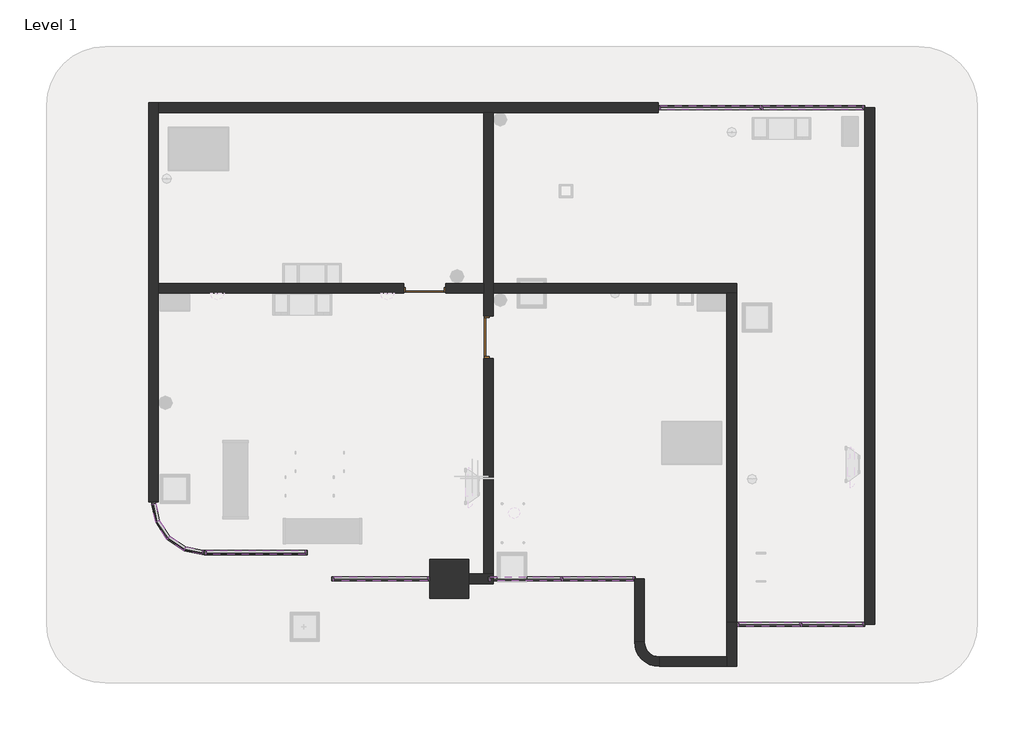
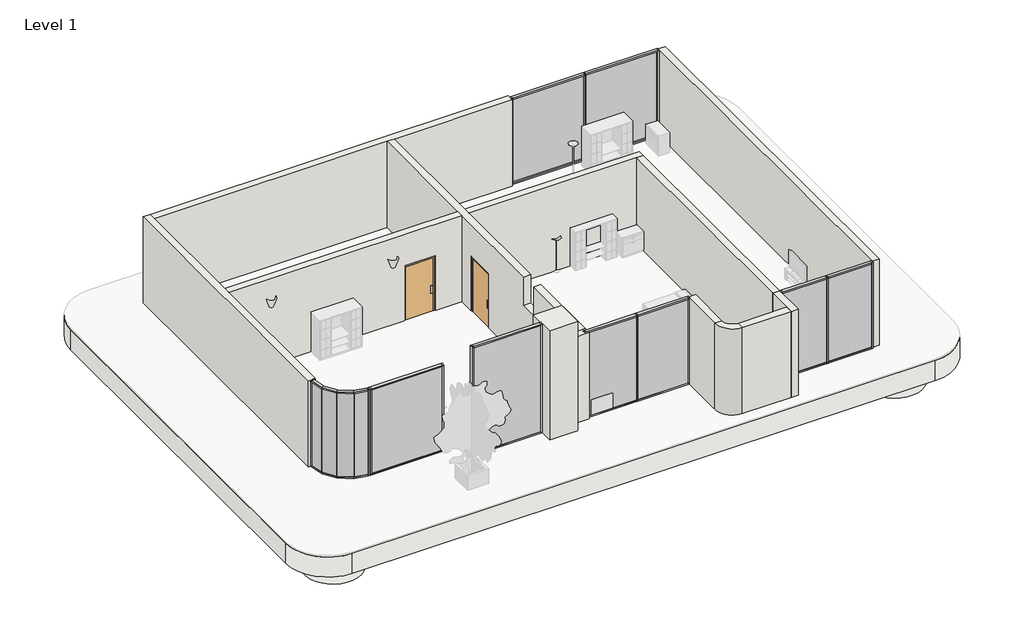
# One storey, part 1 of 2: 39 members, 13 walls, 12 plates, 2 doors, 2 slabs.
"""IFC4 building model written with IfcOpenShell, lengths in millimetres."""

from ifc_helpers import new_model, si_unit, point, frame, frame_2d, origin, origin_with_axes, place, context, project, spatial, polyline, circle_curve, trimmed, segment, composite_curve, outline, extrude, faceted_brep, transform, mapped, element, save
from components import door_bb6275b8, member_c78e4eb6, member_e5c989f4, member_5be86ab4, member_8daf8b49, member_d457d5cf, member_c0191917, member_8659189c, member_c6c1cc64, member_4115b715, member_cd715f5c, member_3783eaa0, system_panel_glazed_b7adf6b9, system_panel_glazed_da3fd9d5, system_panel_glazed_c96b3bd4, system_panel_glazed_89573664, system_panel_glazed_d7bd2e6f, system_panel_glazed_222d0587, system_panel_glazed_285d4db3

model = new_model("IFC4")

# Units and contexts
model_context = context("Model", 3, world=origin())
ifc_project = project(units=[si_unit("LENGTHUNIT", "METRE", prefix="MILLI")], contexts=[model_context])

# Site, building, storey
site = spatial("IfcSite", under=ifc_project)
building = spatial("IfcBuilding", under=site)
storey = spatial("IfcBuildingStorey", under=building, Name="Level 1", Elevation=0.0)

# Doors
placement = place(None, origin())
door_shape = door_bb6275b8(model_context)
element("IfcDoor", 1, ObjectType="Door-Passage-Single-Flush-Dbl_Acting : 48\" x 96\"", at=placement, inside=storey, context=model_context, shape_type="MappedRepresentation", body=[
    mapped(door_shape, transform((-6301.686879, 3653.6091958, 990.6), x_axis=(0.0, 1.0, 0.0), y_axis=(-1.0, 0.0, 0.0), z_axis=(0.0, 0.0, 1.0))),
])
element("IfcDoor", 2, ObjectType="Door-Passage-Single-Flush-Dbl_Acting : 48\" x 96\"", at=placement, inside=storey, context=model_context, shape_type="MappedRepresentation", body=[
    mapped(door_shape, transform((-8289.236879, 5183.9591958, 990.6), x_axis=(-1.0, 0.0, 0.0), y_axis=(0.0, -1.0, 0.0), z_axis=(0.0, 0.0, 1.0))),
])

# Members
member_shape = member_c78e4eb6(model_context)
element("IfcMember", 3, ObjectType="Rectangular Mullion : 2.5\" x 5\" rectangular", at=placement, inside=storey, context=model_context, shape_type="MappedRepresentation", body=[
    mapped(member_shape, transform((1477.063121, -5282.5562261, 4953.0), x_axis=(0.0, 0.0, 1.0), y_axis=(0.0, 1.0, 0.0), z_axis=(-1.0, 0.0, 0.0))),
])
element("IfcMember", 4, ObjectType="Rectangular Mullion : 2.5\" x 5\" rectangular", at=placement, inside=storey, context=model_context, shape_type="MappedRepresentation", body=[
    mapped(member_shape, transform((3437.1390628, -5282.5562261, 4953.0), x_axis=(0.0, 0.0, 1.0), y_axis=(0.0, 1.0, 0.0), z_axis=(-1.0, 0.0, 0.0))),
])
element("IfcMember", 5, ObjectType="Rectangular Mullion : 2.5\" x 5\" rectangular", at=placement, inside=storey, context=model_context, shape_type="MappedRepresentation", body=[
    mapped(member_shape, transform((5333.7150045, -5282.5562261, 990.6), x_axis=(0.0, 0.0, -1.0), y_axis=(0.0, 1.0, 0.0), z_axis=(1.0, 0.0, 0.0))),
])
element("IfcMember", 6, ObjectType="Rectangular Mullion : 2.5\" x 5\" rectangular", at=placement, inside=storey, context=model_context, shape_type="MappedRepresentation", body=[
    mapped(member_shape, transform((3373.6390628, -5282.5562261, 990.6), x_axis=(0.0, 0.0, -1.0), y_axis=(0.0, 1.0, 0.0), z_axis=(1.0, 0.0, 0.0))),
])
member_2_shape = member_e5c989f4(model_context)
element("IfcMember", 7, ObjectType="Rectangular Mullion : 2.5\" x 5\" rectangular", at=placement, inside=storey, context=model_context, shape_type="MappedRepresentation", body=[
    mapped(member_2_shape, transform((3405.3890628, -5282.5562261, 990.6), x_axis=(-1.0, 0.0, 0.0), y_axis=(0.0, 1.0, 0.0), z_axis=(0.0, 0.0, -1.0))),
])
element("IfcMember", 8, ObjectType="Rectangular Mullion : 2.5\" x 5\" rectangular", at=placement, inside=storey, context=model_context, shape_type="MappedRepresentation", body=[
    mapped(member_2_shape, transform((-4022.036879, -3864.7908042, 990.6), x_axis=(-1.0, 0.0, 0.0), y_axis=(0.0, 1.0, 0.0), z_axis=(0.0, 0.0, -1.0))),
])
element("IfcMember", 9, ObjectType="Rectangular Mullion : 2.5\" x 5\" rectangular", at=placement, inside=storey, context=model_context, shape_type="MappedRepresentation", body=[
    mapped(member_2_shape, transform((2184.9997478, 10795.6437739, 990.6), x_axis=(1.0, 0.0, 0.0), y_axis=(0.0, -1.0, 0.0), z_axis=(0.0, 0.0, -1.0))),
])
member_3_shape = member_5be86ab4(model_context)
element("IfcMember", 10, ObjectType="Rectangular Mullion : 2.5\" x 5\" rectangular", at=placement, inside=storey, context=model_context, shape_type="MappedRepresentation", body=[
    mapped(member_3_shape, transform((1413.563121, -5282.5562261, 990.6), x_axis=(-1.0, 0.0, 0.0), y_axis=(0.0, 1.0, 0.0), z_axis=(0.0, 0.0, -1.0))),
])
element("IfcMember", 11, ObjectType="Rectangular Mullion : 2.5\" x 5\" rectangular", at=placement, inside=storey, context=model_context, shape_type="MappedRepresentation", body=[
    mapped(member_3_shape, transform((-6308.036879, -3864.7908042, 990.6), x_axis=(-1.0, 0.0, 0.0), y_axis=(0.0, 1.0, 0.0), z_axis=(0.0, 0.0, -1.0))),
])
element("IfcMember", 12, ObjectType="Rectangular Mullion : 2.5\" x 5\" rectangular", at=placement, inside=storey, context=model_context, shape_type="MappedRepresentation", body=[
    mapped(member_3_shape, transform((5397.2150045, 10795.6437739, 990.6), x_axis=(1.0, 0.0, 0.0), y_axis=(0.0, -1.0, 0.0), z_axis=(0.0, 0.0, -1.0))),
])
element("IfcMember", 13, ObjectType="Rectangular Mullion : 2.5\" x 5\" rectangular", at=placement, inside=storey, context=model_context, shape_type="MappedRepresentation", body=[
    mapped(member_3_shape, transform((-15147.236879, -3051.9908042, 990.6), x_axis=(-1.0, 0.0, 0.0), y_axis=(0.0, 1.0, 0.0), z_axis=(0.0, 0.0, -1.0))),
])
element("IfcMember", 14, ObjectType="Rectangular Mullion : 2.5\" x 5\" rectangular", at=placement, inside=storey, context=model_context, shape_type="MappedRepresentation", body=[
    mapped(member_3_shape, transform((-16724.4155088, -1474.8121743, 990.6), x_axis=(-0.19509032201611579, 0.980785280403233, 0.0), y_axis=(0.980785280403233, 0.19509032201611579, 0.0), z_axis=(0.0, 0.0, -1.0))),
])
element("IfcMember", 15, ObjectType="Rectangular Mullion : 2.5\" x 5\" rectangular", at=placement, inside=storey, context=model_context, shape_type="MappedRepresentation", body=[
    mapped(member_3_shape, transform((5397.2150045, -5282.5562261, 4953.0), x_axis=(1.0, 0.0, 0.0), y_axis=(0.0, 1.0, 0.0), z_axis=(0.0, 0.0, 1.0))),
])
element("IfcMember", 16, ObjectType="Rectangular Mullion : 2.5\" x 5\" rectangular", at=placement, inside=storey, context=model_context, shape_type="MappedRepresentation", body=[
    mapped(member_3_shape, transform((-1736.036879, -3864.7908042, 4953.0), x_axis=(1.0, 0.0, 0.0), y_axis=(0.0, 1.0, 0.0), z_axis=(0.0, 0.0, 1.0))),
])
element("IfcMember", 17, ObjectType="Rectangular Mullion : 2.5\" x 5\" rectangular", at=placement, inside=storey, context=model_context, shape_type="MappedRepresentation", body=[
    mapped(member_3_shape, transform((-1027.2155088, 10795.6437739, 4953.0), x_axis=(-1.0, 0.0, 0.0), y_axis=(0.0, -1.0, 0.0), z_axis=(0.0, 0.0, 1.0))),
])
element("IfcMember", 18, ObjectType="Rectangular Mullion : 2.5\" x 5\" rectangular", at=placement, inside=storey, context=model_context, shape_type="MappedRepresentation", body=[
    mapped(member_3_shape, transform((-11946.836879, -3051.9908042, 4953.0), x_axis=(1.0, 0.0, 0.0), y_axis=(0.0, 1.0, 0.0), z_axis=(0.0, 0.0, 1.0))),
])
element("IfcMember", 19, ObjectType="Rectangular Mullion : 2.5\" x 5\" rectangular", at=placement, inside=storey, context=model_context, shape_type="MappedRepresentation", body=[
    mapped(member_3_shape, transform((-15147.236879, -3051.9908042, 4953.0), x_axis=(0.9807852804032273, -0.19509032201614393, 0.0), y_axis=(0.19509032201614393, 0.9807852804032273, 0.0), z_axis=(0.0, 0.0, 1.0))),
])
member_4_shape = member_8daf8b49(model_context)
element("IfcMember", 20, ObjectType="Rectangular Mullion : 2.5\" x 5\" rectangular", at=placement, inside=storey, context=model_context, shape_type="MappedRepresentation", body=[
    mapped(member_4_shape, transform((-6244.536879, -3864.7908042, 4953.0), x_axis=(0.0, 0.0, 1.0), y_axis=(0.0, 1.0, 0.0), z_axis=(-1.0, 0.0, 0.0))),
])
element("IfcMember", 21, ObjectType="Rectangular Mullion : 2.5\" x 5\" rectangular", at=placement, inside=storey, context=model_context, shape_type="MappedRepresentation", body=[
    mapped(member_4_shape, transform((-3990.286879, -3864.7908042, 4953.0), x_axis=(0.0, 0.0, 1.0), y_axis=(0.0, 1.0, 0.0), z_axis=(-1.0, 0.0, 0.0))),
])
element("IfcMember", 22, ObjectType="Rectangular Mullion : 2.5\" x 5\" rectangular", at=placement, inside=storey, context=model_context, shape_type="MappedRepresentation", body=[
    mapped(member_4_shape, transform((-1799.536879, -3864.7908042, 990.6), x_axis=(0.0, 0.0, -1.0), y_axis=(0.0, 1.0, 0.0), z_axis=(1.0, 0.0, 0.0))),
])
element("IfcMember", 23, ObjectType="Rectangular Mullion : 2.5\" x 5\" rectangular", at=placement, inside=storey, context=model_context, shape_type="MappedRepresentation", body=[
    mapped(member_4_shape, transform((-4053.786879, -3864.7908042, 990.6), x_axis=(0.0, 0.0, -1.0), y_axis=(0.0, 1.0, 0.0), z_axis=(1.0, 0.0, 0.0))),
])
member_5_shape = member_d457d5cf(model_context)
element("IfcMember", 24, ObjectType="Rectangular Mullion : 2.5\" x 5\" rectangular", at=placement, inside=storey, context=model_context, shape_type="MappedRepresentation", body=[
    mapped(member_5_shape, transform((-11121.336879, -3864.7908042, 5994.4), x_axis=(0.0, 0.0, 1.0), y_axis=(0.0, 1.0, 0.0), z_axis=(-1.0, 0.0, 0.0))),
])
element("IfcMember", 25, ObjectType="Rectangular Mullion : 2.5\" x 5\" rectangular", at=placement, inside=storey, context=model_context, shape_type="MappedRepresentation", body=[
    mapped(member_5_shape, transform((-8200.336879, -3864.7908042, 990.6), x_axis=(0.0, 0.0, -1.0), y_axis=(0.0, 1.0, 0.0), z_axis=(1.0, 0.0, 0.0))),
])
member_6_shape = member_c0191917(model_context)
element("IfcMember", 26, ObjectType="Rectangular Mullion : 2.5\" x 5\" rectangular", at=placement, inside=storey, context=model_context, shape_type="MappedRepresentation", body=[
    mapped(member_6_shape, transform((5333.7150045, 10795.6437739, 4953.0), x_axis=(0.0, 0.0, 1.0), y_axis=(0.0, -1.0, 0.0), z_axis=(1.0, 0.0, 0.0))),
])
element("IfcMember", 27, ObjectType="Rectangular Mullion : 2.5\" x 5\" rectangular", at=placement, inside=storey, context=model_context, shape_type="MappedRepresentation", body=[
    mapped(member_6_shape, transform((2153.2497478, 10795.6437739, 4953.0), x_axis=(0.0, 0.0, 1.0), y_axis=(0.0, -1.0, 0.0), z_axis=(1.0, 0.0, 0.0))),
])
element("IfcMember", 28, ObjectType="Rectangular Mullion : 2.5\" x 5\" rectangular", at=placement, inside=storey, context=model_context, shape_type="MappedRepresentation", body=[
    mapped(member_6_shape, transform((-963.7155088, 10795.6437739, 990.6), x_axis=(0.0, 0.0, -1.0), y_axis=(0.0, -1.0, 0.0), z_axis=(-1.0, 0.0, 0.0))),
])
element("IfcMember", 29, ObjectType="Rectangular Mullion : 2.5\" x 5\" rectangular", at=placement, inside=storey, context=model_context, shape_type="MappedRepresentation", body=[
    mapped(member_6_shape, transform((2216.7497478, 10795.6437739, 990.6), x_axis=(0.0, 0.0, -1.0), y_axis=(0.0, -1.0, 0.0), z_axis=(-1.0, 0.0, 0.0))),
])
member_7_shape = member_8659189c(model_context)
element("IfcMember", 30, ObjectType="Rectangular Mullion : 2.5\" x 5\" rectangular", at=placement, inside=storey, context=model_context, shape_type="MappedRepresentation", body=[
    mapped(member_7_shape, transform((-16712.0272734, -1537.0920396, 4953.0), x_axis=(0.0, 0.0, 1.0), y_axis=(0.980785280403233, 0.19509032201611579, 0.0), z_axis=(-0.19509032201611579, 0.980785280403233, 0.0))),
])
member_8_shape = member_c6c1cc64(model_context)
element("IfcMember", 31, ObjectType="Rectangular Mullion : 2.5\" x 5\" rectangular", at=placement, inside=storey, context=model_context, shape_type="MappedRepresentation", body=[
    mapped(member_8_shape, transform((-16262.4705833, -2590.0458786, 990.6), x_axis=(0.0, 0.0, -1.0), y_axis=(0.8314696123025568, 0.5555702330195851, 0.0), z_axis=(0.555570233019585, -0.8314696123025567, 0.0))),
])
element("IfcMember", 32, ObjectType="Rectangular Mullion : 2.5\" x 5\" rectangular", at=placement, inside=storey, context=model_context, shape_type="MappedRepresentation", body=[
    mapped(member_8_shape, transform((-16604.3599342, -2078.3723059, 4953.0), x_axis=(0.0, 0.0, 1.0), y_axis=(0.831469612302557, 0.5555702330195846, 0.0), z_axis=(-0.5555702330195846, 0.831469612302557, 0.0))),
])
member_9_shape = member_4115b715(model_context)
element("IfcMember", 33, ObjectType="Rectangular Mullion : 2.5\" x 5\" rectangular", at=placement, inside=storey, context=model_context, shape_type="MappedRepresentation", body=[
    mapped(member_9_shape, transform((-16604.3599342, -2078.3723059, 990.6), x_axis=(0.0, 0.0, -1.0), y_axis=(0.980785280403233, 0.19509032201611579, 0.0), z_axis=(0.19509032201611579, -0.980785280403233, 0.0))),
])
member_10_shape = member_cd715f5c(model_context)
element("IfcMember", 34, ObjectType="Rectangular Mullion : 2.5\" x 5\" rectangular", at=placement, inside=storey, context=model_context, shape_type="MappedRepresentation", body=[
    mapped(member_10_shape, transform((-11184.836879, -3864.7908042, 990.6), x_axis=(-1.0, 0.0, 0.0), y_axis=(0.0, 1.0, 0.0), z_axis=(0.0, 0.0, -1.0))),
])
element("IfcMember", 35, ObjectType="Rectangular Mullion : 2.5\" x 5\" rectangular", at=placement, inside=storey, context=model_context, shape_type="MappedRepresentation", body=[
    mapped(member_10_shape, transform((-8136.836879, -3864.7908042, 5994.4), x_axis=(1.0, 0.0, 0.0), y_axis=(0.0, 1.0, 0.0), z_axis=(0.0, 0.0, 1.0))),
])
element("IfcMember", 36, ObjectType="Rectangular Mullion : 2.5\" x 5\" rectangular", at=placement, inside=storey, context=model_context, shape_type="MappedRepresentation", body=[
    mapped(member_8_shape, transform((-16262.4705833, -2590.0458786, 4953.0), x_axis=(0.0, 0.0, 1.0), y_axis=(0.5555702330196194, 0.8314696123025339, 0.0), z_axis=(-0.8314696123025338, 0.5555702330196193, 0.0))),
])
element("IfcMember", 37, ObjectType="Rectangular Mullion : 2.5\" x 5\" rectangular", at=placement, inside=storey, context=model_context, shape_type="MappedRepresentation", body=[
    mapped(member_8_shape, transform((-15750.7970105, -2931.9352296, 990.6), x_axis=(0.0, 0.0, -1.0), y_axis=(0.5555702330196189, 0.8314696123025341, 0.0), z_axis=(0.831469612302534, -0.5555702330196188, 0.0))),
])
element("IfcMember", 38, ObjectType="Rectangular Mullion : 2.5\" x 5\" rectangular", at=placement, inside=storey, context=model_context, shape_type="MappedRepresentation", body=[
    mapped(member_7_shape, transform((-15209.5167443, -3039.6025687, 990.6), x_axis=(0.0, 0.0, -1.0), y_axis=(0.19509032201614393, 0.9807852804032273, 0.0), z_axis=(0.9807852804032272, -0.1950903220161439, 0.0))),
])
element("IfcMember", 39, ObjectType="Rectangular Mullion : 2.5\" x 5\" rectangular", at=placement, inside=storey, context=model_context, shape_type="MappedRepresentation", body=[
    mapped(member_9_shape, transform((-15750.7970105, -2931.9352296, 4953.0), x_axis=(0.0, 0.0, 1.0), y_axis=(0.19509032201614393, 0.9807852804032273, 0.0), z_axis=(-0.9807852804032272, 0.1950903220161439, 0.0))),
])
member_11_shape = member_3783eaa0(model_context)
element("IfcMember", 40, ObjectType="Rectangular Mullion : 2.5\" x 5\" rectangular", at=placement, inside=storey, context=model_context, shape_type="MappedRepresentation", body=[
    mapped(member_11_shape, transform((-15083.736879, -3051.9908042, 4953.0), x_axis=(0.0, 0.0, 1.0), y_axis=(0.0, 1.0, 0.0), z_axis=(-1.0, 0.0, 0.0))),
])
element("IfcMember", 41, ObjectType="Rectangular Mullion : 2.5\" x 5\" rectangular", at=placement, inside=storey, context=model_context, shape_type="MappedRepresentation", body=[
    mapped(member_11_shape, transform((-12010.336879, -3051.9908042, 990.6), x_axis=(0.0, 0.0, -1.0), y_axis=(0.0, 1.0, 0.0), z_axis=(1.0, 0.0, 0.0))),
])

# Plates
system_panel_glazed_shape = system_panel_glazed_b7adf6b9(model_context)
element("IfcPlate", 42, ObjectType="System Panel : Glazed", at=placement, inside=storey, context=model_context, shape_type="MappedRepresentation", body=[
    mapped(system_panel_glazed_shape, transform((4385.4270336, -5282.5562261, 1054.1), x_axis=(-1.0, 0.0, 0.0), y_axis=(0.0, -1.0, 0.0), z_axis=(0.0, 0.0, 1.0))),
])
element("IfcPlate", 43, ObjectType="System Panel : Glazed", at=placement, inside=storey, context=model_context, shape_type="MappedRepresentation", body=[
    mapped(system_panel_glazed_shape, transform((2425.3510919, -5282.5562261, 1054.1), x_axis=(-1.0, 0.0, 0.0), y_axis=(0.0, -1.0, 0.0), z_axis=(0.0, 0.0, 1.0))),
])
system_panel_glazed_2_shape = system_panel_glazed_da3fd9d5(model_context)
element("IfcPlate", 44, ObjectType="System Panel : Glazed", at=placement, inside=storey, context=model_context, shape_type="MappedRepresentation", body=[
    mapped(system_panel_glazed_2_shape, transform((-2894.911879, -3864.7908042, 1054.1), x_axis=(-1.0, 0.0, 0.0), y_axis=(0.0, -1.0, 0.0), z_axis=(0.0, 0.0, 1.0))),
])
element("IfcPlate", 45, ObjectType="System Panel : Glazed", at=placement, inside=storey, context=model_context, shape_type="MappedRepresentation", body=[
    mapped(system_panel_glazed_2_shape, transform((-5149.161879, -3864.7908042, 1054.1), x_axis=(-1.0, 0.0, 0.0), y_axis=(0.0, -1.0, 0.0), z_axis=(0.0, 0.0, 1.0))),
])
system_panel_glazed_3_shape = system_panel_glazed_c96b3bd4(model_context)
element("IfcPlate", 46, ObjectType="System Panel : Glazed", at=placement, inside=storey, context=model_context, shape_type="MappedRepresentation", body=[
    mapped(system_panel_glazed_3_shape, transform((594.7671195, 10795.6437739, 1054.1), x_axis=(1.0, 0.0, 0.0), y_axis=(0.0, 1.0, 0.0), z_axis=(0.0, 0.0, 1.0))),
])
element("IfcPlate", 47, ObjectType="System Panel : Glazed", at=placement, inside=storey, context=model_context, shape_type="MappedRepresentation", body=[
    mapped(system_panel_glazed_3_shape, transform((3775.2323762, 10795.6437739, 1054.1), x_axis=(1.0, 0.0, 0.0), y_axis=(0.0, 1.0, 0.0), z_axis=(0.0, 0.0, 1.0))),
])
system_panel_glazed_4_shape = system_panel_glazed_89573664(model_context)
element("IfcPlate", 48, ObjectType="System Panel : Glazed", at=placement, inside=storey, context=model_context, shape_type="MappedRepresentation", body=[
    mapped(system_panel_glazed_4_shape, transform((-15480.1568774, -2985.7688991, 1054.1), x_axis=(-0.9807852804032273, 0.19509032201614393, 0.0), y_axis=(-0.19509032201614393, -0.9807852804032273, 0.0), z_axis=(0.0, 0.0, 1.0))),
])
element("IfcPlate", 49, ObjectType="System Panel : Glazed", at=placement, inside=storey, context=model_context, shape_type="MappedRepresentation", body=[
    mapped(system_panel_glazed_4_shape, transform((-16658.1936038, -1807.7321727, 1054.1), x_axis=(-0.19509032201611579, 0.980785280403233, 0.0), y_axis=(-0.980785280403233, -0.19509032201611579, 0.0), z_axis=(0.0, 0.0, 1.0))),
])
system_panel_glazed_5_shape = system_panel_glazed_d7bd2e6f(model_context)
element("IfcPlate", 50, ObjectType="System Panel : Glazed", at=placement, inside=storey, context=model_context, shape_type="MappedRepresentation", body=[
    mapped(system_panel_glazed_5_shape, transform((-16433.4152587, -2334.2090922, 1054.1), x_axis=(-0.5555702330195851, 0.8314696123025568, 0.0), y_axis=(-0.8314696123025568, -0.5555702330195851, 0.0), z_axis=(0.0, 0.0, 1.0))),
])
element("IfcPlate", 51, ObjectType="System Panel : Glazed", at=placement, inside=storey, context=model_context, shape_type="MappedRepresentation", body=[
    mapped(system_panel_glazed_5_shape, transform((-16006.6337969, -2760.9905541, 1054.1), x_axis=(-0.8314696123025341, 0.5555702330196189, 0.0), y_axis=(-0.5555702330196189, -0.8314696123025341, 0.0), z_axis=(0.0, 0.0, 1.0))),
])
system_panel_glazed_6_shape = system_panel_glazed_222d0587(model_context)
element("IfcPlate", 52, ObjectType="System Panel : Glazed", at=placement, inside=storey, context=model_context, shape_type="MappedRepresentation", body=[
    mapped(system_panel_glazed_6_shape, transform((-9660.836879, -3864.7908042, 1054.1), x_axis=(-1.0, 0.0, 0.0), y_axis=(0.0, -1.0, 0.0), z_axis=(0.0, 0.0, 1.0))),
])
system_panel_glazed_7_shape = system_panel_glazed_285d4db3(model_context)
element("IfcPlate", 53, ObjectType="System Panel : Glazed", at=placement, inside=storey, context=model_context, shape_type="MappedRepresentation", body=[
    mapped(system_panel_glazed_7_shape, transform((-13547.036879, -3051.9908042, 1054.1), x_axis=(-1.0, 0.0, 0.0), y_axis=(0.0, -1.0, 0.0), z_axis=(0.0, 0.0, 1.0))),
])

# Slabs
element("IfcSlab", 54, ObjectType="Generic - 3'", at=placement, inside=storey, context=model_context, shape_type="SweptSolid", body=[
    extrude(outline(composite_curve([segment(trimmed(circle_curve(frame_2d((7073.6150045, 10871.8437739)), 1828.8), [point((7073.6150045, 12700.6437739))], [point((8902.4150045, 10871.8437739))], False, "CARTESIAN"), True, "CONTINUOUS"), segment(polyline([(8902.4150045, 10871.8437739), (8902.4150045, -5282.5562261)]), True, "CONTINUOUS"), segment(trimmed(circle_curve(frame_2d((7073.6150045, -5282.5562261)), 1828.8), [point((8902.4150045, -5282.5562261))], [point((7073.6150045, -7111.3562261))], False, "CARTESIAN"), True, "CONTINUOUS"), segment(polyline([(7073.6150045, -7111.3562261), (-18224.7849955, -7111.3562261)]), True, "CONTINUOUS"), segment(trimmed(circle_curve(frame_2d((-18224.7849955, -5282.5562261)), 1828.8), [point((-18224.7849955, -7111.3562261))], [point((-20053.5849955, -5282.5562261))], False, "CARTESIAN"), True, "CONTINUOUS"), segment(polyline([(-20053.5849955, -5282.5562261), (-20053.5849955, 10871.8437739)]), True, "CONTINUOUS"), segment(trimmed(circle_curve(frame_2d((-18224.7849955, 10871.8437739)), 1828.8), [point((-20053.5849955, 10871.8437739))], [point((-18224.7849955, 12700.6437739))], False, "CARTESIAN"), True, "CONTINUOUS"), segment(polyline([(-18224.7849955, 12700.6437739), (7073.6150045, 12700.6437739)]), True, "CONTINUOUS")], self_intersect=False)), origin_with_axes(), (0.0, 0.0, 1.0), 914.4),
])
element("IfcSlab", 55, ObjectType="Generic - 4'", at=placement, inside=storey, context=model_context, shape_type="SweptSolid", body=[
    extrude(outline(composite_curve([segment(trimmed(circle_curve(frame_2d((6642.5508629, 10443.6424497)), 1219.2), [point((5423.3508629, 10443.6424497))], [point((6642.5508629, 9224.4424497))], False, "CARTESIAN"), True, "CONTINUOUS"), segment(polyline([(6642.5508629, 9224.4424497), (6642.5508629, -3577.1575503)]), True, "CONTINUOUS"), segment(trimmed(circle_curve(frame_2d((6642.5508629, -4796.3575503)), 1219.2), [point((6642.5508629, -3577.1575503))], [point((5423.3508629, -4796.3575503))], False, "CARTESIAN"), True, "CONTINUOUS"), segment(polyline([(5423.3508629, -4796.3575503), (-16522.2491371, -4796.3575503)]), True, "CONTINUOUS"), segment(trimmed(circle_curve(frame_2d((-17741.4491371, -4796.3575503)), 1219.2), [point((-16522.2491371, -4796.3575503))], [point((-17741.4491371, -3577.1575503))], False, "CARTESIAN"), True, "CONTINUOUS"), segment(polyline([(-17741.4491371, -3577.1575503), (-17741.4491371, 9224.4424497)]), True, "CONTINUOUS"), segment(trimmed(circle_curve(frame_2d((-17741.4491371, 10443.6424497)), 1219.2), [point((-17741.4491371, 9224.4424497))], [point((-16522.2491371, 10443.6424497))], False, "CARTESIAN"), True, "CONTINUOUS"), segment(polyline([(-16522.2491371, 10443.6424497), (5423.3508629, 10443.6424497)]), True, "CONTINUOUS")], self_intersect=False)), frame((0.0, 0.0, -1219.2), z_axis=(0.0, 0.0, 1.0), x_axis=(1.0, 0.0, 0.0)), (0.0, 0.0, 1.0), 1219.2),
])

# Walls
element("IfcWall", 56, ObjectType="Generic - 12\"", at=placement, inside=storey, context=model_context, shape_type="Brep", body=[
    faceted_brep([(1108.763121, -5225.9294098, 990.6), (1108.763121, -6292.7294098, 990.6), (1108.763121, -6597.5294098, 990.6), (1108.763121, -6597.5294098, 4953.0), (1108.763121, -6292.7294098, 4953.0), (1108.763121, -5225.9294098, 4953.0), (1413.563121, -5225.9294098, 990.6), (1413.563121, -5225.9294098, 4953.0), (1413.563121, -6597.5294098, 4953.0), (1413.563121, -6597.5294098, 990.6)], [[[0, 1, 2, 3, 4, 5]], [[6, 7, 8, 9]], [[2, 1, 0, 6, 9]], [[5, 4, 3, 8, 7]], [[0, 5, 7, 6]], [[3, 2, 9, 8]]]),
])
element("IfcWall", 57, ObjectType="Generic - 12\"", at=placement, inside=storey, context=model_context, shape_type="SweptSolid", body=[
    extrude(outline(polyline([(-999.436879, -6292.7294098), (1108.763121, -6292.7294098), (1108.763121, -6597.5294098), (-999.436879, -6597.5294098), (-999.436879, -6292.7294098)])), frame((0.0, 0.0, 990.6), z_axis=(0.0, 0.0, 1.0), x_axis=(1.0, 0.0, 0.0)), (0.0, 0.0, 1.0), 3962.4),
])
element("IfcWall", 58, ObjectType="Generic - 12\"", at=placement, inside=storey, context=model_context, shape_type="SweptSolid", body=[
    extrude(outline(polyline([(-1456.636879, -3864.7908042), (-1456.636879, -5835.5294098), (-1761.436879, -5835.5294098), (-1761.436879, -3864.7908042), (-1456.636879, -3864.7908042)])), frame((0.0, 0.0, 990.6), z_axis=(0.0, 0.0, 1.0), x_axis=(1.0, 0.0, 0.0)), (0.0, 0.0, 1.0), 3962.4),
])
element("IfcWall", 59, ObjectType="Generic - 12\"", at=placement, inside=storey, context=model_context, shape_type="SweptSolid", body=[
    extrude(outline(composite_curve([segment(polyline([(-999.436879, -6292.7294098), (-999.436879, -6597.5294098)]), True, "CONTINUOUS"), segment(trimmed(circle_curve(frame_2d((-999.436879, -5835.5294098)), 762.0), [point((-999.436879, -6597.5294098))], [point((-1761.436879, -5835.5294098))], False, "CARTESIAN"), True, "CONTINUOUS"), segment(polyline([(-1761.436879, -5835.5294098), (-1456.636879, -5835.5294098)]), True, "CONTINUOUS"), segment(trimmed(circle_curve(frame_2d((-999.436879, -5835.5294098)), 457.2), [point((-1456.636879, -5835.5294098))], [point((-999.436879, -6292.7294098))], True, "CARTESIAN"), True, "CONTINUOUS")], self_intersect=False)), frame((0.0, 0.0, 990.6), z_axis=(0.0, 0.0, 1.0), x_axis=(1.0, 0.0, 0.0)), (0.0, 0.0, 1.0), 3962.4),
])
element("IfcWall", 60, ObjectType="Generic - 12\"", at=placement, inside=storey, context=model_context, shape_type="Brep", body=[
    faceted_brep([(-6155.636879, -3712.3908042, 990.6), (-6460.436879, -3712.3908042, 990.6), (-6917.636879, -3712.3908042, 990.6), (-6917.636879, -3712.3908042, 4953.0), (-6460.436879, -3712.3908042, 4953.0), (-6155.636879, -3712.3908042, 4953.0), (-6155.636879, -4017.1908042, 990.6), (-6155.636879, -4017.1908042, 4953.0), (-6917.636879, -4017.1908042, 4953.0), (-6917.636879, -4017.1908042, 990.6)], [[[0, 1, 2, 3, 4, 5]], [[6, 7, 8, 9]], [[2, 1, 0, 6, 9]], [[3, 2, 9, 8]], [[5, 4, 3, 8, 7]], [[0, 5, 7, 6]]]),
])
element("IfcWall", 61, ObjectType="Generic - 12\"", at=placement, inside=storey, context=model_context, shape_type="Brep", body=[
    faceted_brep([(-6155.636879, -3712.3908042, 4953.0), (-6155.636879, -3712.3908042, 990.6), (-6155.636879, 2993.2091958, 990.6), (-6155.636879, 2993.2091958, 3530.6), (-6155.636879, 4314.0091958, 3530.6), (-6155.636879, 4314.0091958, 990.6), (-6155.636879, 5025.2091958, 990.6), (-6155.636879, 5330.0091958, 990.6), (-6155.636879, 10643.2437739, 990.6), (-6155.636879, 10643.2437739, 4953.0), (-6155.636879, 5330.0091958, 4953.0), (-6155.636879, 5025.2091958, 4953.0), (-6155.636879, 377.0091958, 4953.0), (-6155.636879, 377.0091958, 3648.2722241), (-6155.636879, -384.9908042, 3648.2722241), (-6155.636879, -384.9908042, 4953.0), (-6460.436879, -3712.3908042, 990.6), (-6460.436879, -3712.3908042, 4953.0), (-6460.436879, -384.9908042, 4953.0), (-6460.436879, -384.9908042, 3648.2722241), (-6460.436879, 377.0091958, 3648.2722241), (-6460.436879, 377.0091958, 4953.0), (-6460.436879, 5025.2091958, 4953.0), (-6460.436879, 5330.0091958, 4953.0), (-6460.436879, 10643.2437739, 4953.0), (-6460.436879, 10643.2437739, 990.6), (-6460.436879, 5330.0091958, 990.6), (-6460.436879, 5025.2091958, 990.6), (-6460.436879, 4314.0091958, 990.6), (-6460.436879, 4314.0091958, 3530.6), (-6460.436879, 2993.2091958, 3530.6), (-6460.436879, 2993.2091958, 990.6)], [[[0, 1, 2, 3, 4, 5, 6, 7, 8, 9, 10, 11, 12, 13, 14, 15]], [[16, 17, 18, 19, 20, 21, 22, 23, 24, 25, 26, 27, 28, 29, 30, 31]], [[1, 16, 31, 2]], [[25, 8, 7, 6, 5, 28, 27, 26]], [[17, 0, 15, 18]], [[9, 24, 23, 22, 21, 12, 11, 10]], [[1, 0, 17, 16]], [[9, 8, 25, 24]], [[4, 29, 28, 5]], [[29, 4, 3, 30]], [[30, 3, 2, 31]], [[14, 19, 18, 15]], [[19, 14, 13, 20]], [[20, 13, 12, 21]]]),
])
element("IfcWall", 62, ObjectType="Generic - 12\"", at=placement, inside=storey, context=model_context, shape_type="Brep", body=[
    faceted_brep([(-6155.636879, 5025.2091958, 990.6), (1108.763121, 5025.2091958, 990.6), (1413.563121, 5025.2091958, 990.6), (1413.563121, 5025.2091958, 4953.0), (1108.763121, 5025.2091958, 4953.0), (-6155.636879, 5025.2091958, 4953.0), (-6155.636879, 5330.0091958, 990.6), (-6155.636879, 5330.0091958, 4953.0), (1413.563121, 5330.0091958, 4953.0), (1413.563121, 5330.0091958, 990.6)], [[[0, 1, 2, 3, 4, 5]], [[6, 7, 8, 9]], [[2, 1, 0, 6, 9]], [[5, 4, 3, 8, 7]], [[0, 5, 7, 6]], [[3, 2, 9, 8]]]),
])
element("IfcWall", 63, ObjectType="Generic - 12\"", at=placement, inside=storey, context=model_context, shape_type="SweptSolid", body=[
    extrude(outline(polyline([(1108.763121, -5225.9294098), (1108.763121, 5025.2091958), (1413.563121, 5025.2091958), (1413.563121, -5225.9294098), (1108.763121, -5225.9294098)])), frame((0.0, 0.0, 990.6), z_axis=(0.0, 0.0, 1.0), x_axis=(1.0, 0.0, 0.0)), (0.0, 0.0, 1.0), 3962.4),
])
element("IfcWall", 64, ObjectType="Generic - 12\"", at=placement, inside=storey, context=model_context, shape_type="SweptSolid", body=[
    extrude(outline(polyline([(4953.0, -6460.436879), (4953.0, -16572.0155088), (990.6, -16572.0155088), (990.6, -8949.636879), (3530.6, -8949.636879), (3530.6, -7628.836879), (990.6, -7628.836879), (990.6, -6460.436879), (4953.0, -6460.436879)])), frame((0.0, 5025.2091958, 0.0), z_axis=(0.0, 1.0, 0.0), x_axis=(0.0, 0.0, 1.0)), (0.0, 0.0, 1.0), 304.8),
])
element("IfcWall", 65, ObjectType="Generic - 12\" yellow", at=placement, inside=storey, context=model_context, shape_type="Brep", body=[
    faceted_brep([(-16572.0155088, -1474.8121743, 990.6), (-16572.0155088, 5025.2091958, 990.6), (-16572.0155088, 5330.0091958, 990.6), (-16572.0155088, 10643.2437739, 990.6), (-16572.0155088, 10948.0437739, 990.6), (-16572.0155088, 10948.0437739, 4953.0), (-16572.0155088, 10643.2437739, 4953.0), (-16572.0155088, 5330.0091958, 4953.0), (-16572.0155088, 5025.2091958, 4953.0), (-16572.0155088, -1474.8121743, 4953.0), (-16876.8155088, -1474.8121743, 990.6), (-16876.8155088, -1474.8121743, 4953.0), (-16876.8155088, 10948.0437739, 4953.0), (-16876.8155088, 10948.0437739, 990.6)], [[[0, 1, 2, 3, 4, 5, 6, 7, 8, 9]], [[10, 11, 12, 13]], [[4, 3, 2, 1, 0, 10, 13]], [[9, 8, 7, 6, 5, 12, 11]], [[0, 9, 11, 10]], [[5, 4, 13, 12]]]),
])
element("IfcWall", 66, ObjectType="Generic - 12\" yellow", at=placement, inside=storey, context=model_context, shape_type="SweptSolid", body=[
    extrude(outline(polyline([(5702.0150045, 10795.6437739), (5702.0150045, -5282.5562261), (5397.2150045, -5282.5562261), (5397.2150045, 10795.6437739), (5702.0150045, 10795.6437739)])), frame((0.0, 0.0, 990.6), z_axis=(0.0, 0.0, 1.0), x_axis=(1.0, 0.0, 0.0)), (0.0, 0.0, 1.0), 3962.4),
])
element("IfcWall", 67, ObjectType="Generic - 12\" yellow", at=placement, inside=storey, context=model_context, shape_type="Brep", body=[
    faceted_brep([(-16572.0155088, 10643.2437739, 990.6), (-6460.436879, 10643.2437739, 990.6), (-6155.636879, 10643.2437739, 990.6), (-1027.2155088, 10643.2437739, 990.6), (-1027.2155088, 10643.2437739, 4953.0), (-6155.636879, 10643.2437739, 4953.0), (-6460.436879, 10643.2437739, 4953.0), (-16572.0155088, 10643.2437739, 4953.0), (-16572.0155088, 10948.0437739, 990.6), (-16572.0155088, 10948.0437739, 4953.0), (-1027.2155088, 10948.0437739, 4953.0), (-1027.2155088, 10948.0437739, 990.6)], [[[0, 1, 2, 3, 4, 5, 6, 7]], [[8, 9, 10, 11]], [[3, 2, 1, 0, 8, 11]], [[4, 3, 11, 10]], [[7, 6, 5, 4, 10, 9]], [[0, 7, 9, 8]]]),
])
element("IfcWall", 68, ObjectType="Generic - 7'", at=placement, inside=storey, context=model_context, shape_type="Brep", body=[
    faceted_brep([(-6917.636879, -3255.1908042, 990.6), (-8136.836879, -3255.1908042, 990.6), (-8136.836879, -3255.1908042, 5994.4), (-6917.636879, -3255.1908042, 5994.4), (-6917.636879, -4474.3908042, 990.6), (-6917.636879, -4474.3908042, 5994.4), (-8136.836879, -4474.3908042, 5994.4), (-8136.836879, -4474.3908042, 990.6), (-6917.636879, -3712.3908042, 990.6), (-6917.636879, -4017.1908042, 990.6)], [[[0, 1, 2, 3]], [[4, 5, 6, 7]], [[1, 0, 8, 9, 4, 7]], [[2, 1, 7, 6]], [[3, 2, 6, 5]], [[0, 3, 5, 4, 9, 8]]]),
])

save(model, "model.ifc")

# Revit data of these elements
# Type "Door-Passage-Single-Flush-Dbl_Acting : 48\" x 96\""
#   Type Mark = "8"
#   Assembly Code = "B2030200"
#   Analytic Construction = "Wooden"
#   Thickness = 0' - 1 3/4"
#   Thermal Resistance (R) = 2.5876 (h·ft²·°F)/BTU
#   Swing Angle [instance default] = 45.00°
#   Strike Height = 3' - 4"
#   Rough Width [instance default] = 4' - 4"
#   Rough Height [instance default] = 8' - 4"
#   MF Opening Height [instance default] = 0' - 4"
#   MF Opening Width [instance default] = 0' - 4"
#   Inset Calculate [instance default] = 0' - 4"
#   Masonry Inset [instance default] = 0' - 1"
#   Height = 8' - 0"
#   Width = 4' - 0"
#   Heat Transfer Coefficient (U) = 0.3865 BTU/(h·ft²·°F)
#   Masonry Frame Depth = 0' - 5 3/4"
#   Masonry Frame [instance default] = yes
#   Function = 1
#   Dry Wall Frame [instance default] = no
#   Panel Material = Wood - Birch
#   Frame Material = Metal - Paint Finish - Grey
#   Door Handle Material = Aluminum
#   Visual Light Transmittance = 0
#   Solar Heat Gain Coefficient = 0
#   Wall Closure = (empty or 0)
# Type "Rectangular Mullion : 2.5\" x 5\" rectangular"
#   built-in parameter 1007304 = 0.416667 (stored number, unit not read)
#   built-in parameter 1007301 = 0.104167 (stored number, unit not read)
#   built-in parameter 1007300 = 0.104167 (stored number, unit not read)
# Type "System Panel : Glazed"
#   Construction Type Id = "GSP4R"
#   Analytic Construction = "1/8 in Pilkington single glazing"
#   Visual Light Transmittance = 0.9
#   Solar Heat Gain Coefficient = 0.86
#   Heat Transfer Coefficient (U) = 1.18115 BTU/(h·ft²·°F)
# Type "Generic - 3'"
#   Assembly Code = "B1010"
#   Function = 0
#   Layers, outside or top first: 3' - 0" "Parking Stripe" (function 1)
# Type "Generic - 4'"
#   Assembly Code = "B1010"
#   Function = 0
#   Layers, outside or top first: 4' - 0" "Parking Stripe" (function 1)
# Type "Generic - 12\""
#   Assembly Code = "B2010"
#   Layers, outside or top first: 1' - 0" "Parking Stripe" (function 1)
# Type "Generic - 12\" yellow"
#   Assembly Code = "B2010"
#   Layers, outside or top first: 1' - 0" "Door - Frame" (function 1)
# Type "Generic - 7'"
#   Assembly Code = "B2010"
#   Layers, outside or top first: 4' - 0" "Parking Stripe" (function 1)
# Elements 1, 2 (IfcDoor, "Door-Passage-Single-Flush-Dbl_Acting : 48\" x 96\"")
#   Swing Angle = 45.00°
#   Rough Width = 4' - 4"
#   Rough Height = 8' - 4"
#   Masonry Inset = 0' - 1"
#   MF Opening Width = 0' - 4"
#   MF Opening Height = 0' - 4"
#   Inset Calculate = 0' - 4"
#   Masonry Frame = yes
#   Dry Wall Frame = no
#   Phase Created = New Construction
#   Materials on its faces: "Aluminum", "Metal - Paint Finish - Grey", "Wood - Birch"
# Elements 3, 4, 5, 6, 7, 8, 9, 10, 11, 12, 13, 14, 15, 16, 17, 18, 19, 20, 21, 22, 23, 24, 25, 26, 27, 28, 29, 30, 31, 32, 33, 34, 35, 36, 37, 38, 39, 40, 41 (IfcMember, "Rectangular Mullion : 2.5\" x 5\" rectangular")
#   Phase Created = New Construction
#   Materials on its faces: "Iron, Ductile"
# Elements 42, 43, 44, 45, 46, 47, 48, 49, 50, 51, 52, 53 (IfcPlate, "System Panel : Glazed")
#   Phase Created = New Construction
#   Materials on its faces: "Glass"
# Element 54 (IfcSlab, "Generic - 3'")
#   Height Offset From Level = 3' - 0"
#   Phase Created = New Construction
#   Materials on its faces: "Parking Stripe"
# Element 55 (IfcSlab, "Generic - 4'")
#   Height Offset From Level = 0' - 0"
#   Phase Created = New Construction
#   Materials on its faces: "Parking Stripe"
# Element 56 (IfcWall, "Generic - 12\"")
#   built-in parameter 1001111 = 3' - 3"
#   Top Offset = 0' - 0"
#   Base Offset = 3' - 3"
#   Unconnected Height = 13' - 0"
#   wall height = 13' - 0"
#   Phase Created = New Construction
#   Base Constraint = Level 1
#   Materials on its faces: "Parking Stripe"
# Elements 57, 58, 60, 61, 63, 64 (IfcWall, "Generic - 12\"")
#   built-in parameter 1001111 = 3' - 3"
#   Top Offset = 0' - 0"
#   Base Offset = 3' - 3"
#   Unconnected Height = 13' - 0"
#   wall height = 13' - 0"
#   Phase Created = New Construction
#   Base Constraint = Level 1
#   Materials on its faces: "Parking Stripe", "Door - Frame"
# Element 59 (IfcWall, "Generic - 12\"")
#   built-in parameter 1001111 = 3' - 3"
#   Top Offset = 0' - 0"
#   Base Offset = 3' - 3"
#   Unconnected Height = 13' - 0"
#   wall height = 13' - 0"
#   Phase Created = New Construction
#   Materials on its faces: "Parking Stripe", "Door - Frame"
# Element 62 (IfcWall, "Generic - 12\"")
#   built-in parameter 1001111 = 3' - 3"
#   Top Offset = 0' - 0"
#   Base Offset = 3' - 3"
#   Unconnected Height = 13' - 0"
#   wall height = 13' - 0"
#   Phase Created = New Construction
#   Base Constraint = Level 1
#   Materials on its faces: "Door - Frame", "Parking Stripe"
# Elements 65, 67 (IfcWall, "Generic - 12\" yellow")
#   built-in parameter 1001111 = 3' - 3"
#   Top Offset = 0' - 0"
#   Base Offset = 3' - 3"
#   Unconnected Height = 13' - 0"
#   wall height = 13' - 0"
#   Phase Created = New Construction
#   Base Constraint = Level 1
#   Materials on its faces: "Door - Frame", "Parking Stripe"
# Element 66 (IfcWall, "Generic - 12\" yellow")
#   built-in parameter 1001111 = 3' - 3"
#   Top Offset = 0' - 0"
#   Base Offset = 3' - 3"
#   Unconnected Height = 13' - 0"
#   wall height = 13' - 0"
#   Phase Created = New Construction
#   Base Constraint = Level 1
#   Materials on its faces: "Parking Stripe", "Door - Frame"
# Element 68 (IfcWall, "Generic - 7'")
#   built-in parameter 1001111 = 3' - 3"
#   Top Offset = 0' - 0"
#   Base Offset = 3' - 3"
#   Unconnected Height = 16' - 5"
#   wall height = 16' - 5"
#   Phase Created = New Construction
#   Base Constraint = Level 1
#   Materials on its faces: "Parking Stripe", "Door - Frame"
# Materials
#   "Wood - Birch": class "Wood", colour RGB 166 116 52, transparency 0, Cost = 0
#   "Metal - Paint Finish - Grey": class "Paint", colour RGB 104 104 104, transparency 0, Cost = 0
#   "Aluminum": class "Metal", colour RGB 247 247 247, transparency 0, Description = "Aluminum 6061", Cost = 0
#   "Parking Stripe": class "Paint", colour RGB 250 250 91, transparency 0, Cost = 0
#   "Door - Frame": colour RGB 118 70 51, transparency 0, Cost = 0
#   "Iron, Ductile": class "Metal", colour RGB 0 0 0, transparency 0, Description = "Ductile cast iron", Cost = 0
#   "Glass": class "Glass", colour RGB 0 128 192, transparency 0.75, Description = "Soda Lime Glass", Cost = 0
